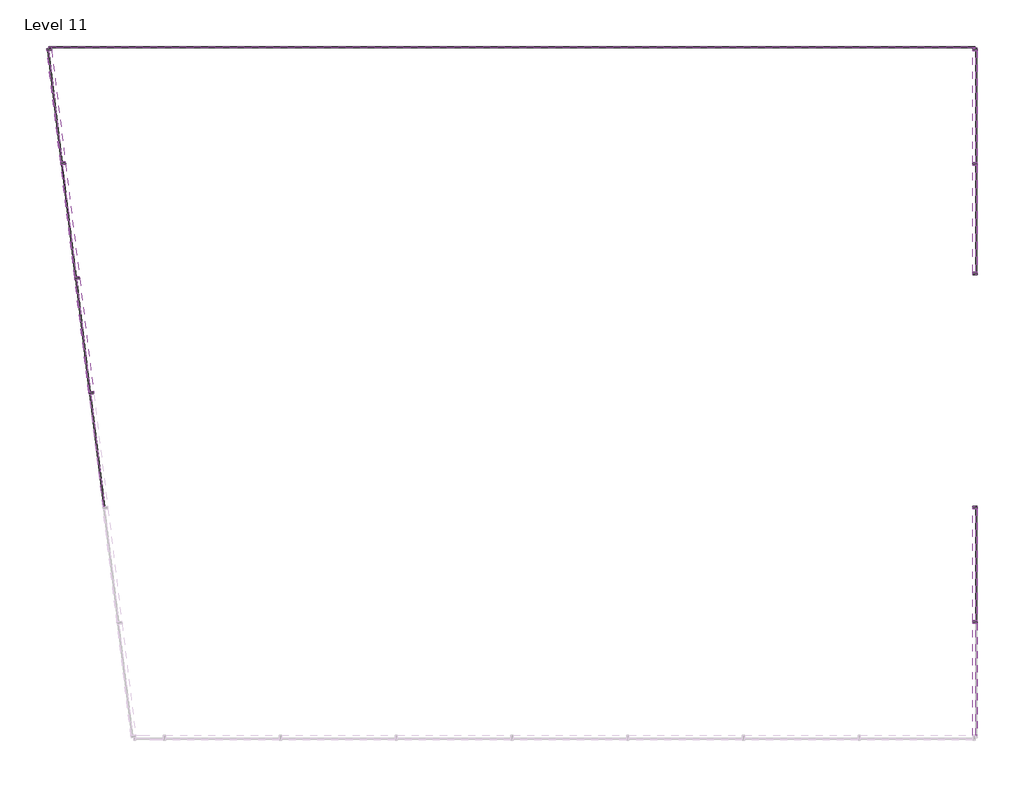
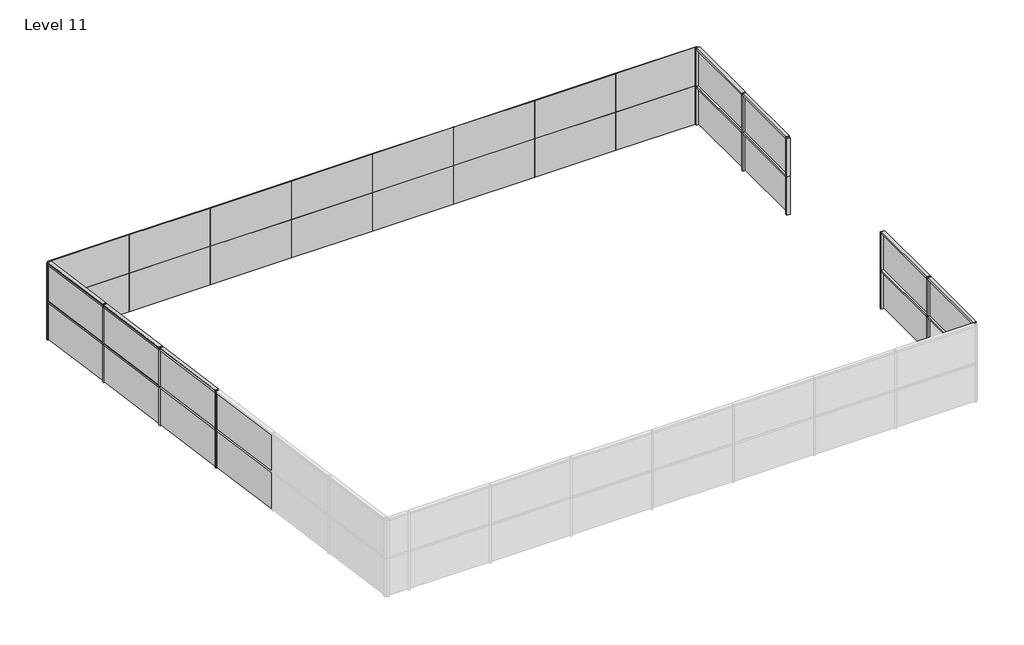
# One storey, part 2 of 2: 46 members, 39 plates.
"""IFC4 building model written with IfcOpenShell, lengths in millimetres."""

from ifc_helpers import new_model, si_unit, origin, place, context, project, spatial, transform, mapped, element, save
from components import member_daa7a266, member_82905deb, member_19d0a4ec, member_8cef0660, member_db480205, member_4491d118, member_46bdb8c2, system_panel_glazed_1e57f9bb, system_panel_glazed_37f15d2e, system_panel_glazed_3620f98e, system_panel_glazed_e46d4b42, system_panel_glazed_2a6c68b7, system_panel_glazed_d483336f

model = new_model("IFC4")

# Units and contexts
model_context = context("Model", 3, world=origin())
ifc_project = project(units=[si_unit("LENGTHUNIT", "METRE", prefix="MILLI")], contexts=[model_context])

# Site, building, storey
site = spatial("IfcSite", under=ifc_project)
building = spatial("IfcBuilding", under=site)
storey = spatial("IfcBuildingStorey", under=building, Name="Level 11", Elevation=30480.0)

# Members
placement = place(None, origin())
member_shape = member_daa7a266(model_context)
element("IfcMember", 1, ObjectType="Rectangular Mullion : 2.5\" x 5\" rectangular", at=placement, inside=storey, context=model_context, shape_type="MappedRepresentation", body=[
    mapped(member_shape, transform((-10113.8959567, 8178.7803212, 33528.0), x_axis=(0.0, 0.0, 1.0), y_axis=(-0.9925461516413222, -0.12186934340514625, 0.0), z_axis=(0.12186934340514625, -0.9925461516413222, 0.0))),
])
member_2_shape = member_82905deb(model_context)
element("IfcMember", 2, ObjectType="Rectangular Mullion : 2.5\" x 5\" rectangular", at=placement, inside=storey, context=model_context, shape_type="MappedRepresentation", body=[
    mapped(member_2_shape, transform((-9367.1110876, 2096.7056405, 33528.0), x_axis=(-0.1218693434051459, 0.9925461516413222, 0.0), y_axis=(-0.9925461516413222, -0.1218693434051459, 0.0), z_axis=(0.0, 0.0, 1.0))),
])
element("IfcMember", 3, ObjectType="Rectangular Mullion : 2.5\" x 5\" rectangular", at=placement, inside=storey, context=model_context, shape_type="MappedRepresentation", body=[
    mapped(member_2_shape, transform((-9738.5688463, 5121.9863107, 33528.0), x_axis=(-0.1218693434051459, 0.9925461516413222, 0.0), y_axis=(-0.9925461516413222, -0.1218693434051459, 0.0), z_axis=(0.0, 0.0, 1.0))),
])
element("IfcMember", 4, ObjectType="Rectangular Mullion : 2.5\" x 5\" rectangular", at=placement, inside=storey, context=model_context, shape_type="MappedRepresentation", body=[
    mapped(member_2_shape, transform((-10110.026605, 8147.2669809, 33528.0), x_axis=(-0.1218693434051459, 0.9925461516413222, 0.0), y_axis=(-0.9925461516413222, -0.1218693434051459, 0.0), z_axis=(0.0, 0.0, 1.0))),
])
member_3_shape = member_19d0a4ec(model_context)
element("IfcMember", 5, ObjectType="Rectangular Mullion : 2.5\" x 5\" rectangular", at=placement, inside=storey, context=model_context, shape_type="MappedRepresentation", body=[
    mapped(member_3_shape, transform((-10113.8959567, 8178.7803212, 32004.0), x_axis=(0.0, 0.0, 1.0), y_axis=(-0.9925461516413223, -0.12186934340514552, 0.0), z_axis=(0.1218693434051455, -0.9925461516413222, 0.0))),
])
element("IfcMember", 6, ObjectType="Rectangular Mullion : 2.5\" x 5\" rectangular", at=placement, inside=storey, context=model_context, shape_type="MappedRepresentation", body=[
    mapped(member_3_shape, transform((-10113.8959567, 8178.7803212, 32004.0), x_axis=(0.0, 0.0, 1.0), y_axis=(-0.9925461516413222, -0.12186934340514599, 0.0), z_axis=(0.12186934340514599, -0.9925461516413222, 0.0))),
])
element("IfcMember", 7, ObjectType="Rectangular Mullion : 2.5\" x 5\" rectangular", at=placement, inside=storey, context=model_context, shape_type="MappedRepresentation", body=[
    mapped(member_3_shape, transform((-10113.8959567, 8178.7803212, 33528.0), x_axis=(0.0, 0.0, 1.0), y_axis=(-0.9925461516413222, -0.12186934340514599, 0.0), z_axis=(0.12186934340514599, -0.9925461516413222, 0.0))),
])
element("IfcMember", 8, ObjectType="Rectangular Mullion : 2.5\" x 5\" rectangular", at=placement, inside=storey, context=model_context, shape_type="MappedRepresentation", body=[
    mapped(member_3_shape, transform((13902.5156363, -946.6363705, 32004.0), x_axis=(0.0, 0.0, 1.0), y_axis=(1.0, 0.0, 0.0), z_axis=(0.0, 1.0, 0.0))),
])
element("IfcMember", 9, ObjectType="Rectangular Mullion : 2.5\" x 5\" rectangular", at=placement, inside=storey, context=model_context, shape_type="MappedRepresentation", body=[
    mapped(member_3_shape, transform((13902.5156363, -3962.8863708, 32004.0), x_axis=(0.0, 0.0, 1.0), y_axis=(1.0, 0.0, 0.0), z_axis=(0.0, 1.0, 0.0))),
])
element("IfcMember", 10, ObjectType="Rectangular Mullion : 2.5\" x 5\" rectangular", at=placement, inside=storey, context=model_context, shape_type="MappedRepresentation", body=[
    mapped(member_3_shape, transform((13902.5156363, -946.6363705, 33528.0), x_axis=(0.0, 0.0, 1.0), y_axis=(1.0, 0.0, 0.0), z_axis=(0.0, 1.0, 0.0))),
])
element("IfcMember", 11, ObjectType="Rectangular Mullion : 2.5\" x 5\" rectangular", at=placement, inside=storey, context=model_context, shape_type="MappedRepresentation", body=[
    mapped(member_3_shape, transform((13902.5156363, -3962.8863708, 33528.0), x_axis=(0.0, 0.0, 1.0), y_axis=(1.0, 0.0, 0.0), z_axis=(0.0, 1.0, 0.0))),
])
element("IfcMember", 12, ObjectType="Rectangular Mullion : 2.5\" x 5\" rectangular", at=placement, inside=storey, context=model_context, shape_type="MappedRepresentation", body=[
    mapped(member_3_shape, transform((13902.5156363, 11109.0476508, 32004.0), x_axis=(0.0, 0.0, 1.0), y_axis=(1.0, 0.0, 0.0), z_axis=(0.0, 1.0, 0.0))),
])
element("IfcMember", 13, ObjectType="Rectangular Mullion : 2.5\" x 5\" rectangular", at=placement, inside=storey, context=model_context, shape_type="MappedRepresentation", body=[
    mapped(member_3_shape, transform((13902.5156363, 11109.0476508, 33528.0), x_axis=(0.0, 0.0, 1.0), y_axis=(1.0, 0.0, 0.0), z_axis=(0.0, 1.0, 0.0))),
])
member_4_shape = member_8cef0660(model_context)
element("IfcMember", 14, ObjectType="Rectangular Mullion : 2.5\" x 5\" rectangular", at=placement, inside=storey, context=model_context, shape_type="MappedRepresentation", body=[
    mapped(member_4_shape, transform((-9370.9804393, 2128.2189808, 32004.0), x_axis=(0.0, 0.0, 1.0), y_axis=(-0.9925461516413222, -0.12186934340514592, 0.0), z_axis=(0.12186934340514592, -0.9925461516413222, 0.0))),
])
element("IfcMember", 15, ObjectType="Rectangular Mullion : 2.5\" x 5\" rectangular", at=placement, inside=storey, context=model_context, shape_type="MappedRepresentation", body=[
    mapped(member_4_shape, transform((-9742.438198, 5153.499651, 32004.0), x_axis=(0.0, 0.0, 1.0), y_axis=(-0.9925461516413222, -0.12186934340514602, 0.0), z_axis=(0.12186934340514602, -0.9925461516413222, 0.0))),
])
element("IfcMember", 16, ObjectType="Rectangular Mullion : 2.5\" x 5\" rectangular", at=placement, inside=storey, context=model_context, shape_type="MappedRepresentation", body=[
    mapped(member_4_shape, transform((-9370.9804393, 2128.2189808, 32004.0), x_axis=(0.0, 0.0, 1.0), y_axis=(-0.9925461516413223, -0.12186934340514566, 0.0), z_axis=(0.12186934340514566, -0.9925461516413223, 0.0))),
])
element("IfcMember", 17, ObjectType="Rectangular Mullion : 2.5\" x 5\" rectangular", at=placement, inside=storey, context=model_context, shape_type="MappedRepresentation", body=[
    mapped(member_4_shape, transform((-9742.438198, 5153.499651, 32004.0), x_axis=(0.0, 0.0, 1.0), y_axis=(-0.9925461516413222, -0.12186934340514602, 0.0), z_axis=(0.12186934340514602, -0.9925461516413222, 0.0))),
])
element("IfcMember", 18, ObjectType="Rectangular Mullion : 2.5\" x 5\" rectangular", at=placement, inside=storey, context=model_context, shape_type="MappedRepresentation", body=[
    mapped(member_4_shape, transform((-9370.9804393, 2128.2189808, 33528.0), x_axis=(0.0, 0.0, 1.0), y_axis=(-0.9925461516413222, -0.12186934340514599, 0.0), z_axis=(0.12186934340514599, -0.9925461516413222, 0.0))),
])
element("IfcMember", 19, ObjectType="Rectangular Mullion : 2.5\" x 5\" rectangular", at=placement, inside=storey, context=model_context, shape_type="MappedRepresentation", body=[
    mapped(member_4_shape, transform((-9742.438198, 5153.499651, 33528.0), x_axis=(0.0, 0.0, 1.0), y_axis=(-0.9925461516413222, -0.12186934340514566, 0.0), z_axis=(0.12186934340514566, -0.9925461516413222, 0.0))),
])
member_5_shape = member_db480205(model_context)
element("IfcMember", 20, ObjectType="Rectangular Mullion : 2.5\" x 5\" rectangular", at=placement, inside=storey, context=model_context, shape_type="MappedRepresentation", body=[
    mapped(member_5_shape, transform((-9370.9804393, 2128.2189808, 33528.0), x_axis=(0.0, 0.0, 1.0), y_axis=(-0.9925461516413222, -0.12186934340514592, 0.0), z_axis=(0.12186934340514592, -0.9925461516413222, 0.0))),
])
element("IfcMember", 21, ObjectType="Rectangular Mullion : 2.5\" x 5\" rectangular", at=placement, inside=storey, context=model_context, shape_type="MappedRepresentation", body=[
    mapped(member_5_shape, transform((-9742.438198, 5153.499651, 33528.0), x_axis=(0.0, 0.0, 1.0), y_axis=(-0.9925461516413222, -0.1218693434051457, 0.0), z_axis=(0.1218693434051457, -0.9925461516413222, 0.0))),
])
element("IfcMember", 22, ObjectType="Rectangular Mullion : 2.5\" x 5\" rectangular", at=placement, inside=storey, context=model_context, shape_type="MappedRepresentation", body=[
    mapped(member_2_shape, transform((-9367.1110876, 2096.7056405, 32004.0), x_axis=(-0.1218693434051459, 0.9925461516413222, 0.0), y_axis=(-0.9925461516413222, -0.1218693434051459, 0.0), z_axis=(0.0, 0.0, 1.0))),
])
element("IfcMember", 23, ObjectType="Rectangular Mullion : 2.5\" x 5\" rectangular", at=placement, inside=storey, context=model_context, shape_type="MappedRepresentation", body=[
    mapped(member_2_shape, transform((-9738.5688463, 5121.9863107, 32004.0), x_axis=(-0.1218693434051459, 0.9925461516413222, 0.0), y_axis=(-0.9925461516413222, -0.1218693434051459, 0.0), z_axis=(0.0, 0.0, 1.0))),
])
element("IfcMember", 24, ObjectType="Rectangular Mullion : 2.5\" x 5\" rectangular", at=placement, inside=storey, context=model_context, shape_type="MappedRepresentation", body=[
    mapped(member_2_shape, transform((-10110.026605, 8147.2669809, 32004.0), x_axis=(-0.1218693434051459, 0.9925461516413222, 0.0), y_axis=(-0.9925461516413222, -0.1218693434051459, 0.0), z_axis=(0.0, 0.0, 1.0))),
])
element("IfcMember", 25, ObjectType="Rectangular Mullion : 2.5\" x 5\" rectangular", at=placement, inside=storey, context=model_context, shape_type="MappedRepresentation", body=[
    mapped(member_2_shape, transform((-9367.1110876, 2096.7056405, 32004.0), x_axis=(-0.1218693434051459, 0.9925461516413222, 0.0), y_axis=(-0.9925461516413222, -0.1218693434051459, 0.0), z_axis=(0.0, 0.0, 1.0))),
])
element("IfcMember", 26, ObjectType="Rectangular Mullion : 2.5\" x 5\" rectangular", at=placement, inside=storey, context=model_context, shape_type="MappedRepresentation", body=[
    mapped(member_2_shape, transform((-9367.1110876, 2096.7056405, 33528.0), x_axis=(-0.1218693434051459, 0.9925461516413222, 0.0), y_axis=(-0.9925461516413222, -0.1218693434051459, 0.0), z_axis=(0.0, 0.0, 1.0))),
])
element("IfcMember", 27, ObjectType="Rectangular Mullion : 2.5\" x 5\" rectangular", at=placement, inside=storey, context=model_context, shape_type="MappedRepresentation", body=[
    mapped(member_2_shape, transform((-9738.5688463, 5121.9863107, 32004.0), x_axis=(-0.1218693434051459, 0.9925461516413222, 0.0), y_axis=(-0.9925461516413222, -0.1218693434051459, 0.0), z_axis=(0.0, 0.0, 1.0))),
])
element("IfcMember", 28, ObjectType="Rectangular Mullion : 2.5\" x 5\" rectangular", at=placement, inside=storey, context=model_context, shape_type="MappedRepresentation", body=[
    mapped(member_2_shape, transform((-9738.5688463, 5121.9863107, 33528.0), x_axis=(-0.1218693434051459, 0.9925461516413222, 0.0), y_axis=(-0.9925461516413222, -0.1218693434051459, 0.0), z_axis=(0.0, 0.0, 1.0))),
])
element("IfcMember", 29, ObjectType="Rectangular Mullion : 2.5\" x 5\" rectangular", at=placement, inside=storey, context=model_context, shape_type="MappedRepresentation", body=[
    mapped(member_2_shape, transform((-10110.026605, 8147.2669809, 32004.0), x_axis=(-0.1218693434051459, 0.9925461516413222, 0.0), y_axis=(-0.9925461516413222, -0.1218693434051459, 0.0), z_axis=(0.0, 0.0, 1.0))),
])
element("IfcMember", 30, ObjectType="Rectangular Mullion : 2.5\" x 5\" rectangular", at=placement, inside=storey, context=model_context, shape_type="MappedRepresentation", body=[
    mapped(member_2_shape, transform((-10110.026605, 8147.2669809, 33528.0), x_axis=(-0.1218693434051459, 0.9925461516413222, 0.0), y_axis=(-0.9925461516413222, -0.1218693434051459, 0.0), z_axis=(0.0, 0.0, 1.0))),
])
element("IfcMember", 31, ObjectType="Rectangular Mullion : 2.5\" x 5\" rectangular", at=placement, inside=storey, context=model_context, shape_type="MappedRepresentation", body=[
    mapped(member_2_shape, transform((13902.5156363, -3931.1363708, 32004.0), x_axis=(0.0, -1.0, 0.0), y_axis=(1.0, 0.0, 0.0), z_axis=(0.0, 0.0, 1.0))),
])
element("IfcMember", 32, ObjectType="Rectangular Mullion : 2.5\" x 5\" rectangular", at=placement, inside=storey, context=model_context, shape_type="MappedRepresentation", body=[
    mapped(member_2_shape, transform((13902.5156363, -3931.1363708, 33528.0), x_axis=(0.0, -1.0, 0.0), y_axis=(1.0, 0.0, 0.0), z_axis=(0.0, 0.0, 1.0))),
])
element("IfcMember", 33, ObjectType="Rectangular Mullion : 2.5\" x 5\" rectangular", at=placement, inside=storey, context=model_context, shape_type="MappedRepresentation", body=[
    mapped(member_2_shape, transform((13902.5156363, 8124.5476505, 32004.0), x_axis=(0.0, -1.0, 0.0), y_axis=(1.0, 0.0, 0.0), z_axis=(0.0, 0.0, 1.0))),
])
element("IfcMember", 34, ObjectType="Rectangular Mullion : 2.5\" x 5\" rectangular", at=placement, inside=storey, context=model_context, shape_type="MappedRepresentation", body=[
    mapped(member_2_shape, transform((13902.5156363, 8124.5476505, 33528.0), x_axis=(0.0, -1.0, 0.0), y_axis=(1.0, 0.0, 0.0), z_axis=(0.0, 0.0, 1.0))),
])
member_6_shape = member_4491d118(model_context)
element("IfcMember", 35, ObjectType="Rectangular Mullion : 2.5\" x 5\" rectangular", at=placement, inside=storey, context=model_context, shape_type="MappedRepresentation", body=[
    mapped(member_6_shape, transform((-10481.4843637, 11172.5476508, 33528.0), x_axis=(-0.1218693434051459, 0.9925461516413222, 0.0), y_axis=(-0.9925461516413222, -0.1218693434051459, 0.0), z_axis=(0.0, 0.0, 1.0))),
])
element("IfcMember", 36, ObjectType="Rectangular Mullion : 2.5\" x 5\" rectangular", at=placement, inside=storey, context=model_context, shape_type="MappedRepresentation", body=[
    mapped(member_6_shape, transform((13902.5156363, -883.1363705, 30480.0), x_axis=(0.0, 1.0, 0.0), y_axis=(1.0, 0.0, 0.0), z_axis=(0.0, 0.0, -1.0))),
])
element("IfcMember", 37, ObjectType="Rectangular Mullion : 2.5\" x 5\" rectangular", at=placement, inside=storey, context=model_context, shape_type="MappedRepresentation", body=[
    mapped(member_6_shape, transform((13902.5156363, -883.1363705, 32004.0), x_axis=(0.0, 1.0, 0.0), y_axis=(1.0, 0.0, 0.0), z_axis=(0.0, 0.0, -1.0))),
])
element("IfcMember", 38, ObjectType="Rectangular Mullion : 2.5\" x 5\" rectangular", at=placement, inside=storey, context=model_context, shape_type="MappedRepresentation", body=[
    mapped(member_6_shape, transform((13902.5156363, 11172.5476508, 30480.0), x_axis=(0.0, 1.0, 0.0), y_axis=(1.0, 0.0, 0.0), z_axis=(0.0, 0.0, -1.0))),
])
element("IfcMember", 39, ObjectType="Rectangular Mullion : 2.5\" x 5\" rectangular", at=placement, inside=storey, context=model_context, shape_type="MappedRepresentation", body=[
    mapped(member_6_shape, transform((13902.5156363, 11172.5476508, 32004.0), x_axis=(0.0, 1.0, 0.0), y_axis=(1.0, 0.0, 0.0), z_axis=(0.0, 0.0, -1.0))),
])
element("IfcMember", 40, ObjectType="Rectangular Mullion : 2.5\" x 5\" rectangular", at=placement, inside=storey, context=model_context, shape_type="MappedRepresentation", body=[
    mapped(member_6_shape, transform((-10481.4843637, 11172.5476508, 32004.0), x_axis=(-0.1218693434051459, 0.9925461516413222, 0.0), y_axis=(-0.9925461516413222, -0.1218693434051459, 0.0), z_axis=(0.0, 0.0, 1.0))),
])
element("IfcMember", 41, ObjectType="Rectangular Mullion : 2.5\" x 5\" rectangular", at=placement, inside=storey, context=model_context, shape_type="MappedRepresentation", body=[
    mapped(member_6_shape, transform((-10481.4843637, 11172.5476508, 32004.0), x_axis=(-0.1218693434051459, 0.9925461516413222, 0.0), y_axis=(-0.9925461516413222, -0.1218693434051459, 0.0), z_axis=(0.0, 0.0, 1.0))),
])
element("IfcMember", 42, ObjectType="Rectangular Mullion : 2.5\" x 5\" rectangular", at=placement, inside=storey, context=model_context, shape_type="MappedRepresentation", body=[
    mapped(member_6_shape, transform((-10481.4843637, 11172.5476508, 33528.0), x_axis=(-0.1218693434051459, 0.9925461516413222, 0.0), y_axis=(-0.9925461516413222, -0.1218693434051459, 0.0), z_axis=(0.0, 0.0, 1.0))),
])
element("IfcMember", 43, ObjectType="Rectangular Mullion : 2.5\" x 5\" rectangular", at=placement, inside=storey, context=model_context, shape_type="MappedRepresentation", body=[
    mapped(member_6_shape, transform((13902.5156363, 5212.8636295, 32004.0), x_axis=(0.0, -1.0, 0.0), y_axis=(1.0, 0.0, 0.0), z_axis=(0.0, 0.0, 1.0))),
])
element("IfcMember", 44, ObjectType="Rectangular Mullion : 2.5\" x 5\" rectangular", at=placement, inside=storey, context=model_context, shape_type="MappedRepresentation", body=[
    mapped(member_6_shape, transform((13902.5156363, 5212.8636295, 33528.0), x_axis=(0.0, -1.0, 0.0), y_axis=(1.0, 0.0, 0.0), z_axis=(0.0, 0.0, 1.0))),
])
member_7_shape = member_46bdb8c2(model_context)
element("IfcMember", 45, ObjectType="Rectangular Mullion : 2.5\" x 5\" rectangular", at=placement, inside=storey, context=model_context, shape_type="MappedRepresentation", body=[
    mapped(member_7_shape, transform((13902.5156363, 8092.7976505, 32004.0), x_axis=(0.0, 0.0, 1.0), y_axis=(1.0, 0.0, 0.0), z_axis=(0.0, 1.0, 0.0))),
])
element("IfcMember", 46, ObjectType="Rectangular Mullion : 2.5\" x 5\" rectangular", at=placement, inside=storey, context=model_context, shape_type="MappedRepresentation", body=[
    mapped(member_7_shape, transform((13902.5156363, 8092.7976505, 33528.0), x_axis=(0.0, 0.0, 1.0), y_axis=(1.0, 0.0, 0.0), z_axis=(0.0, 1.0, 0.0))),
])

# Plates
system_panel_glazed_shape = system_panel_glazed_1e57f9bb(model_context)
element("IfcPlate", 47, ObjectType="System Panel : Glazed", at=placement, inside=storey, context=model_context, shape_type="MappedRepresentation", body=[
    mapped(system_panel_glazed_shape, transform((-8957.4843636, 11172.5476508, 30480.0), x_axis=(1.0, 0.0, 0.0), y_axis=(0.0, 1.0, 0.0), z_axis=(0.0, 0.0, 1.0))),
])
element("IfcPlate", 48, ObjectType="System Panel : Glazed", at=placement, inside=storey, context=model_context, shape_type="MappedRepresentation", body=[
    mapped(system_panel_glazed_shape, transform((-5909.4843634, 11172.5476508, 30480.0), x_axis=(1.0, 0.0, 0.0), y_axis=(0.0, 1.0, 0.0), z_axis=(0.0, 0.0, 1.0))),
])
element("IfcPlate", 49, ObjectType="System Panel : Glazed", at=placement, inside=storey, context=model_context, shape_type="MappedRepresentation", body=[
    mapped(system_panel_glazed_shape, transform((-2861.4843634, 11172.5476508, 30480.0), x_axis=(1.0, 0.0, 0.0), y_axis=(0.0, 1.0, 0.0), z_axis=(0.0, 0.0, 1.0))),
])
element("IfcPlate", 50, ObjectType="System Panel : Glazed", at=placement, inside=storey, context=model_context, shape_type="MappedRepresentation", body=[
    mapped(system_panel_glazed_shape, transform((186.5156366, 11172.5476508, 30480.0), x_axis=(1.0, 0.0, 0.0), y_axis=(0.0, 1.0, 0.0), z_axis=(0.0, 0.0, 1.0))),
])
element("IfcPlate", 51, ObjectType="System Panel : Glazed", at=placement, inside=storey, context=model_context, shape_type="MappedRepresentation", body=[
    mapped(system_panel_glazed_shape, transform((3234.5156366, 11172.5476508, 30480.0), x_axis=(1.0, 0.0, 0.0), y_axis=(0.0, 1.0, 0.0), z_axis=(0.0, 0.0, 1.0))),
])
element("IfcPlate", 52, ObjectType="System Panel : Glazed", at=placement, inside=storey, context=model_context, shape_type="MappedRepresentation", body=[
    mapped(system_panel_glazed_shape, transform((6282.5156366, 11172.5476508, 30480.0), x_axis=(1.0, 0.0, 0.0), y_axis=(0.0, 1.0, 0.0), z_axis=(0.0, 0.0, 1.0))),
])
element("IfcPlate", 53, ObjectType="System Panel : Glazed", at=placement, inside=storey, context=model_context, shape_type="MappedRepresentation", body=[
    mapped(system_panel_glazed_shape, transform((9330.5156366, 11172.5476508, 30480.0), x_axis=(1.0, 0.0, 0.0), y_axis=(0.0, 1.0, 0.0), z_axis=(0.0, 0.0, 1.0))),
])
element("IfcPlate", 54, ObjectType="System Panel : Glazed", at=placement, inside=storey, context=model_context, shape_type="MappedRepresentation", body=[
    mapped(system_panel_glazed_shape, transform((12378.5156364, 11172.5476508, 30480.0), x_axis=(1.0, 0.0, 0.0), y_axis=(0.0, 1.0, 0.0), z_axis=(0.0, 0.0, 1.0))),
])
element("IfcPlate", 55, ObjectType="System Panel : Glazed", at=placement, inside=storey, context=model_context, shape_type="MappedRepresentation", body=[
    mapped(system_panel_glazed_shape, transform((-8957.4843636, 11172.5476508, 32004.0), x_axis=(1.0, 0.0, 0.0), y_axis=(0.0, 1.0, 0.0), z_axis=(0.0, 0.0, 1.0))),
])
element("IfcPlate", 56, ObjectType="System Panel : Glazed", at=placement, inside=storey, context=model_context, shape_type="MappedRepresentation", body=[
    mapped(system_panel_glazed_shape, transform((-5909.4843634, 11172.5476508, 32004.0), x_axis=(1.0, 0.0, 0.0), y_axis=(0.0, 1.0, 0.0), z_axis=(0.0, 0.0, 1.0))),
])
element("IfcPlate", 57, ObjectType="System Panel : Glazed", at=placement, inside=storey, context=model_context, shape_type="MappedRepresentation", body=[
    mapped(system_panel_glazed_shape, transform((-2861.4843634, 11172.5476508, 32004.0), x_axis=(1.0, 0.0, 0.0), y_axis=(0.0, 1.0, 0.0), z_axis=(0.0, 0.0, 1.0))),
])
element("IfcPlate", 58, ObjectType="System Panel : Glazed", at=placement, inside=storey, context=model_context, shape_type="MappedRepresentation", body=[
    mapped(system_panel_glazed_shape, transform((186.5156366, 11172.5476508, 32004.0), x_axis=(1.0, 0.0, 0.0), y_axis=(0.0, 1.0, 0.0), z_axis=(0.0, 0.0, 1.0))),
])
element("IfcPlate", 59, ObjectType="System Panel : Glazed", at=placement, inside=storey, context=model_context, shape_type="MappedRepresentation", body=[
    mapped(system_panel_glazed_shape, transform((3234.5156366, 11172.5476508, 32004.0), x_axis=(1.0, 0.0, 0.0), y_axis=(0.0, 1.0, 0.0), z_axis=(0.0, 0.0, 1.0))),
])
element("IfcPlate", 60, ObjectType="System Panel : Glazed", at=placement, inside=storey, context=model_context, shape_type="MappedRepresentation", body=[
    mapped(system_panel_glazed_shape, transform((6282.5156366, 11172.5476508, 32004.0), x_axis=(1.0, 0.0, 0.0), y_axis=(0.0, 1.0, 0.0), z_axis=(0.0, 0.0, 1.0))),
])
element("IfcPlate", 61, ObjectType="System Panel : Glazed", at=placement, inside=storey, context=model_context, shape_type="MappedRepresentation", body=[
    mapped(system_panel_glazed_shape, transform((9330.5156366, 11172.5476508, 32004.0), x_axis=(1.0, 0.0, 0.0), y_axis=(0.0, 1.0, 0.0), z_axis=(0.0, 0.0, 1.0))),
])
element("IfcPlate", 62, ObjectType="System Panel : Glazed", at=placement, inside=storey, context=model_context, shape_type="MappedRepresentation", body=[
    mapped(system_panel_glazed_shape, transform((12378.5156364, 11172.5476508, 32004.0), x_axis=(1.0, 0.0, 0.0), y_axis=(0.0, 1.0, 0.0), z_axis=(0.0, 0.0, 1.0))),
])
system_panel_glazed_2_shape = system_panel_glazed_37f15d2e(model_context)
element("IfcPlate", 63, ObjectType="System Panel : Glazed", at=placement, inside=storey, context=model_context, shape_type="MappedRepresentation", body=[
    mapped(system_panel_glazed_2_shape, transform((-10293.8208085, 9644.1506457, 32035.75), x_axis=(-0.1218693434051459, 0.9925461516413222, 0.0), y_axis=(-0.9925461516413222, -0.1218693434051459, 0.0), z_axis=(0.0, 0.0, 1.0))),
])
system_panel_glazed_3_shape = system_panel_glazed_3620f98e(model_context)
element("IfcPlate", 64, ObjectType="System Panel : Glazed", at=placement, inside=storey, context=model_context, shape_type="MappedRepresentation", body=[
    mapped(system_panel_glazed_3_shape, transform((-9181.3822083, 584.0653054, 32035.75), x_axis=(-0.1218693434051459, 0.9925461516413222, 0.0), y_axis=(-0.9925461516413222, -0.1218693434051459, 0.0), z_axis=(0.0, 0.0, 1.0))),
])
element("IfcPlate", 65, ObjectType="System Panel : Glazed", at=placement, inside=storey, context=model_context, shape_type="MappedRepresentation", body=[
    mapped(system_panel_glazed_3_shape, transform((-9552.839967, 3609.3459756, 32035.75), x_axis=(-0.1218693434051459, 0.9925461516413222, 0.0), y_axis=(-0.9925461516413222, -0.1218693434051459, 0.0), z_axis=(0.0, 0.0, 1.0))),
])
element("IfcPlate", 66, ObjectType="System Panel : Glazed", at=placement, inside=storey, context=model_context, shape_type="MappedRepresentation", body=[
    mapped(system_panel_glazed_3_shape, transform((-9924.2977257, 6634.6266458, 32035.75), x_axis=(-0.1218693434051459, 0.9925461516413222, 0.0), y_axis=(-0.9925461516413222, -0.1218693434051459, 0.0), z_axis=(0.0, 0.0, 1.0))),
])
system_panel_glazed_4_shape = system_panel_glazed_e46d4b42(model_context)
element("IfcPlate", 67, ObjectType="System Panel : Glazed", at=placement, inside=storey, context=model_context, shape_type="MappedRepresentation", body=[
    mapped(system_panel_glazed_4_shape, transform((-10293.8208085, 9644.1506457, 30511.75), x_axis=(-0.1218693434051459, 0.9925461516413222, 0.0), y_axis=(-0.9925461516413222, -0.1218693434051459, 0.0), z_axis=(0.0, 0.0, 1.0))),
])
element("IfcPlate", 68, ObjectType="System Panel : Glazed", at=placement, inside=storey, context=model_context, shape_type="MappedRepresentation", body=[
    mapped(system_panel_glazed_4_shape, transform((-10293.8208085, 9644.1506457, 30511.75), x_axis=(-0.1218693434051459, 0.9925461516413222, 0.0), y_axis=(-0.9925461516413222, -0.1218693434051459, 0.0), z_axis=(0.0, 0.0, 1.0))),
])
element("IfcPlate", 69, ObjectType="System Panel : Glazed", at=placement, inside=storey, context=model_context, shape_type="MappedRepresentation", body=[
    mapped(system_panel_glazed_4_shape, transform((-10293.8208085, 9644.1506457, 32035.75), x_axis=(-0.1218693434051459, 0.9925461516413222, 0.0), y_axis=(-0.9925461516413222, -0.1218693434051459, 0.0), z_axis=(0.0, 0.0, 1.0))),
])
element("IfcPlate", 70, ObjectType="System Panel : Glazed", at=placement, inside=storey, context=model_context, shape_type="MappedRepresentation", body=[
    mapped(system_panel_glazed_4_shape, transform((13902.5156363, -2423.0113706, 30511.75), x_axis=(0.0, -1.0, 0.0), y_axis=(1.0, 0.0, 0.0), z_axis=(0.0, 0.0, 1.0))),
])
element("IfcPlate", 71, ObjectType="System Panel : Glazed", at=placement, inside=storey, context=model_context, shape_type="MappedRepresentation", body=[
    mapped(system_panel_glazed_4_shape, transform((13902.5156363, -2423.0113706, 32035.75), x_axis=(0.0, -1.0, 0.0), y_axis=(1.0, 0.0, 0.0), z_axis=(0.0, 0.0, 1.0))),
])
element("IfcPlate", 72, ObjectType="System Panel : Glazed", at=placement, inside=storey, context=model_context, shape_type="MappedRepresentation", body=[
    mapped(system_panel_glazed_4_shape, transform((13902.5156363, -5439.2613706, 32035.75), x_axis=(0.0, -1.0, 0.0), y_axis=(1.0, 0.0, 0.0), z_axis=(0.0, 0.0, 1.0))),
])
element("IfcPlate", 73, ObjectType="System Panel : Glazed", at=placement, inside=storey, context=model_context, shape_type="MappedRepresentation", body=[
    mapped(system_panel_glazed_4_shape, transform((13902.5156363, 9632.6726506, 30511.75), x_axis=(0.0, -1.0, 0.0), y_axis=(1.0, 0.0, 0.0), z_axis=(0.0, 0.0, 1.0))),
])
element("IfcPlate", 74, ObjectType="System Panel : Glazed", at=placement, inside=storey, context=model_context, shape_type="MappedRepresentation", body=[
    mapped(system_panel_glazed_4_shape, transform((13902.5156363, 9632.6726506, 32035.75), x_axis=(0.0, -1.0, 0.0), y_axis=(1.0, 0.0, 0.0), z_axis=(0.0, 0.0, 1.0))),
])
system_panel_glazed_5_shape = system_panel_glazed_2a6c68b7(model_context)
element("IfcPlate", 75, ObjectType="System Panel : Glazed", at=placement, inside=storey, context=model_context, shape_type="MappedRepresentation", body=[
    mapped(system_panel_glazed_5_shape, transform((-9181.3822083, 584.0653054, 30511.75), x_axis=(-0.1218693434051459, 0.9925461516413222, 0.0), y_axis=(-0.9925461516413222, -0.1218693434051459, 0.0), z_axis=(0.0, 0.0, 1.0))),
])
element("IfcPlate", 76, ObjectType="System Panel : Glazed", at=placement, inside=storey, context=model_context, shape_type="MappedRepresentation", body=[
    mapped(system_panel_glazed_5_shape, transform((-9552.839967, 3609.3459756, 30511.75), x_axis=(-0.1218693434051459, 0.9925461516413222, 0.0), y_axis=(-0.9925461516413222, -0.1218693434051459, 0.0), z_axis=(0.0, 0.0, 1.0))),
])
element("IfcPlate", 77, ObjectType="System Panel : Glazed", at=placement, inside=storey, context=model_context, shape_type="MappedRepresentation", body=[
    mapped(system_panel_glazed_5_shape, transform((-9924.2977257, 6634.6266458, 30511.75), x_axis=(-0.1218693434051459, 0.9925461516413222, 0.0), y_axis=(-0.9925461516413222, -0.1218693434051459, 0.0), z_axis=(0.0, 0.0, 1.0))),
])
element("IfcPlate", 78, ObjectType="System Panel : Glazed", at=placement, inside=storey, context=model_context, shape_type="MappedRepresentation", body=[
    mapped(system_panel_glazed_5_shape, transform((-9181.3822083, 584.0653054, 30511.75), x_axis=(-0.1218693434051459, 0.9925461516413222, 0.0), y_axis=(-0.9925461516413222, -0.1218693434051459, 0.0), z_axis=(0.0, 0.0, 1.0))),
])
element("IfcPlate", 79, ObjectType="System Panel : Glazed", at=placement, inside=storey, context=model_context, shape_type="MappedRepresentation", body=[
    mapped(system_panel_glazed_5_shape, transform((-9552.839967, 3609.3459756, 30511.75), x_axis=(-0.1218693434051459, 0.9925461516413222, 0.0), y_axis=(-0.9925461516413222, -0.1218693434051459, 0.0), z_axis=(0.0, 0.0, 1.0))),
])
element("IfcPlate", 80, ObjectType="System Panel : Glazed", at=placement, inside=storey, context=model_context, shape_type="MappedRepresentation", body=[
    mapped(system_panel_glazed_5_shape, transform((-9924.2977257, 6634.6266458, 30511.75), x_axis=(-0.1218693434051459, 0.9925461516413222, 0.0), y_axis=(-0.9925461516413222, -0.1218693434051459, 0.0), z_axis=(0.0, 0.0, 1.0))),
])
element("IfcPlate", 81, ObjectType="System Panel : Glazed", at=placement, inside=storey, context=model_context, shape_type="MappedRepresentation", body=[
    mapped(system_panel_glazed_5_shape, transform((-9181.3822083, 584.0653054, 32035.75), x_axis=(-0.1218693434051459, 0.9925461516413222, 0.0), y_axis=(-0.9925461516413222, -0.1218693434051459, 0.0), z_axis=(0.0, 0.0, 1.0))),
])
element("IfcPlate", 82, ObjectType="System Panel : Glazed", at=placement, inside=storey, context=model_context, shape_type="MappedRepresentation", body=[
    mapped(system_panel_glazed_5_shape, transform((-9552.839967, 3609.3459756, 32035.75), x_axis=(-0.1218693434051459, 0.9925461516413222, 0.0), y_axis=(-0.9925461516413222, -0.1218693434051459, 0.0), z_axis=(0.0, 0.0, 1.0))),
])
element("IfcPlate", 83, ObjectType="System Panel : Glazed", at=placement, inside=storey, context=model_context, shape_type="MappedRepresentation", body=[
    mapped(system_panel_glazed_5_shape, transform((-9924.2977257, 6634.6266458, 32035.75), x_axis=(-0.1218693434051459, 0.9925461516413222, 0.0), y_axis=(-0.9925461516413222, -0.1218693434051459, 0.0), z_axis=(0.0, 0.0, 1.0))),
])
system_panel_glazed_6_shape = system_panel_glazed_d483336f(model_context)
element("IfcPlate", 84, ObjectType="System Panel : Glazed", at=placement, inside=storey, context=model_context, shape_type="MappedRepresentation", body=[
    mapped(system_panel_glazed_6_shape, transform((13902.5156363, 6684.58064, 30511.75), x_axis=(0.0, -1.0, 0.0), y_axis=(1.0, 0.0, 0.0), z_axis=(0.0, 0.0, 1.0))),
])
element("IfcPlate", 85, ObjectType="System Panel : Glazed", at=placement, inside=storey, context=model_context, shape_type="MappedRepresentation", body=[
    mapped(system_panel_glazed_6_shape, transform((13902.5156363, 6684.58064, 32035.75), x_axis=(0.0, -1.0, 0.0), y_axis=(1.0, 0.0, 0.0), z_axis=(0.0, 0.0, 1.0))),
])

save(model, "model.ifc")

# Revit data of these elements
# Type "Rectangular Mullion : 2.5\" x 5\" rectangular"
#   built-in parameter 1007304 = 0.416667 (stored number, unit not read)
#   built-in parameter 1007301 = 0.104167 (stored number, unit not read)
#   built-in parameter 1007300 = 0.104167 (stored number, unit not read)
# Type "System Panel : Glazed"
#   Construction Type Id = "GSP4R"
#   Analytic Construction = "1/8 in Pilkington single glazing"
#   Visual Light Transmittance = 0.9
#   Solar Heat Gain Coefficient = 0.86
#   Heat Transfer Coefficient (U) = 1.18115 BTU/(h·ft²·°F)
#   Define Thermal Properties by = 1
# Elements 1, 2, 3, 4, 5, 6, 7, 8, 9, 10, 11, 12, 13, 14, 15, 16, 17, 18, 19, 20, 21, 22, 23, 24, 25, 26, 27, 28, 29, 30, 31, 32, 33, 34, 35, 36, 37, 38, 39, 40, 41, 42, 43, 44, 45, 46 (IfcMember, "Rectangular Mullion : 2.5\" x 5\" rectangular")
#   Phase Created = New Construction
#   Materials on its faces: "Aluminum"
# Elements 47, 48, 49, 50, 51, 52, 53, 54, 55, 56, 57, 58, 59, 60, 61, 62, 63, 64, 65, 66, 67, 68, 69, 70, 71, 72, 73, 74, 75, 76, 77, 78, 79, 80, 81, 82, 83, 84, 85 (IfcPlate, "System Panel : Glazed")
#   Phase Created = New Construction
#   Materials on its faces: "Glass"
# Materials
#   "Aluminum": class "Metal", colour RGB 247 247 247, transparency 0, Description = "Aluminum 6061", Cost = 0
#   "Glass": class "Glass", colour RGB 0 128 192, transparency 0.75, Description = "Soda Lime Glass", Cost = 0
